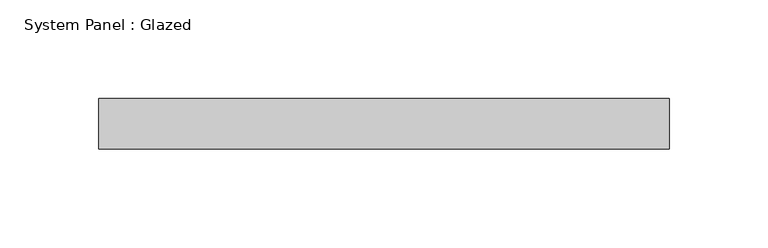
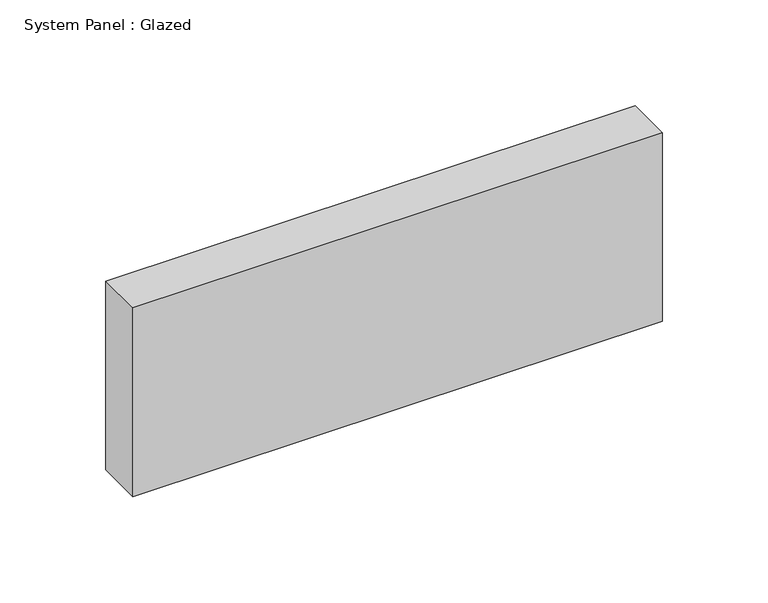
"""IFC4 building model written with IfcOpenShell, lengths in millimetres: plate geometry, System Panel : Glazed."""

from ifc_helpers import new_model, si_unit, origin, origin_with_axes, place, context, project, spatial, polyline, outline, extrude, source, transform, mapped, element, save


def system_panel_glazed_822b3193(model_context):
    return source(origin(), model_context, "Body", "SweptSolid", [
        extrude(outline(polyline([(144.1160334, 19.05), (-144.1160334, 19.05), (-144.1160334, 44.45), (144.1160334, 44.45), (144.1160334, 19.05)])), origin_with_axes(), (0.0, 0.0, 1.0), 108.6326151),
    ])


if __name__ == "__main__":
    model = new_model("IFC4")
    model_context = context("Model", 3, world=origin())
    ifc_project = project(units=[si_unit("LENGTHUNIT", "METRE", prefix="MILLI")], contexts=[model_context])
    site = spatial("IfcSite", under=ifc_project)
    building = spatial("IfcBuilding", under=site)
    placement = place(None, origin())
    system_panel_glazed_shape = system_panel_glazed_822b3193(model_context)
    element("IfcPlate", 1, ObjectType="System Panel : Glazed", at=placement, inside=building, context=model_context, shape_type="MappedRepresentation", body=[
        mapped(system_panel_glazed_shape, transform((0.0, 0.0, 0.0), x_axis=(1.0, 0.0, 0.0), y_axis=(0.0, 1.0, 0.0), z_axis=(0.0, 0.0, 1.0))),
    ])
    save(model, "model.ifc")

# Revit data of these elements
# Type "System Panel : Glazed"
#   Construction Type Id = "GSP4R"
#   Analytic Construction = "1/8 in Pilkington single glazing"
#   Visual Light Transmittance = 0.9
#   Solar Heat Gain Coefficient = 0.86
#   Heat Transfer Coefficient (U) = 1.18115 BTU/(h·ft²·°F)
#   Define Thermal Properties by = 1
# Element 1 (IfcPlate, "System Panel : Glazed")
#   Materials on its faces: "Glass"
# Materials
#   "Glass": class "Glass", colour RGB 0 128 192, transparency 0.75, Description = "Soda Lime Glass", Cost = 0
